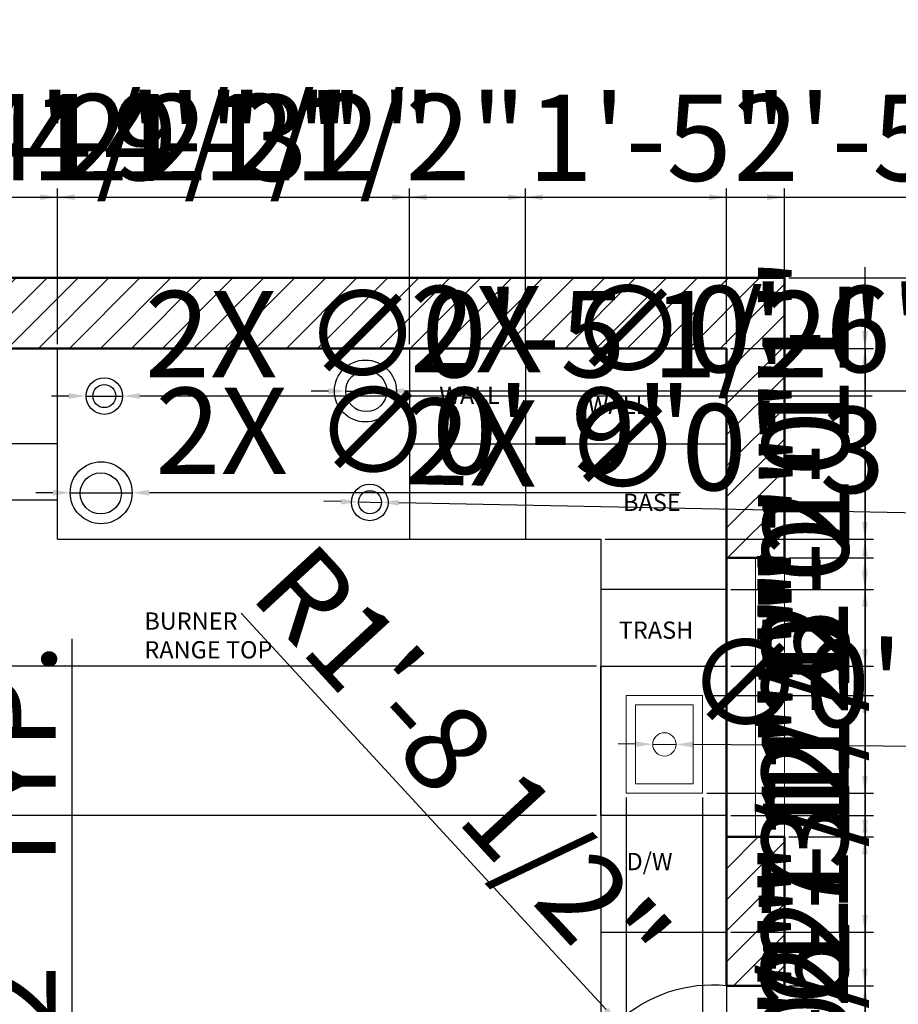
# Model space of a CAD drawing. Units: inches. Extents: x 1545 to 1898, y 1984 to 2198.
# Tile 3 of 4: x 1649 to 1777, y 2055 to 2198. Entities that reach past the tile are written whole.
import ezdxf

# ---------------------------------------------------------------- set-up
doc = ezdxf.new("R2010")
doc.units = ezdxf.units.IN
for name, color, linetype, lineweight in [('A-ANNO-DIMS', 2, 'Continuous', 18), ('A-ANNO-TEXT', 7, 'Continuous', 18), ('A-DOOR', 4, 'Continuous', 25), ('A-EQPM', 9, 'Continuous', 25), ('A-FLOR-CASE', 8, 'Continuous', 25), ('A-FLOR-FIXT', 8, 'Continuous', 18), ('A-GLAZ', 4, 'Continuous', 18), ('A-WALL', 7, 'Continuous', 50), ('A-WALL-PATT', 252, 'Continuous', 13)]:
    doc.layers.add(name, color=color, linetype=linetype, lineweight=lineweight)
doc.styles.get("Standard").update_dxf_attribs({"font": 'arial.ttf'})
doc.dimstyles.new('ISO-25', dxfattribs={"dimtxt": 12.5, "dimasz": 2.5, "dimexe": 1.25, "dimexo": 0.625, "dimtad": 1, "dimdec": 0, "dimlunit": 3, "dimtxsty": 'Standard', "dimcen": 2.5, "dimadec": 0, "dimazin": 0, "dimtfac": 1, "dimtdec": 0, "dimtmove": 0, "dimatfit": 3, "dimfxl": 1, "dimarcsym": 0})

# ---------------------------------------------------------------- blocks, each defined once
blk = doc.blocks.new('*D5')
at = {"layer": 'A-ANNO-DIMS', "color": 0, "lineweight": -2, "transparency": 16777216}
for p, q in [((1760.62, 2160.51), (1812.93, 2160.51)), ((1811.68, 2158.01), (1811.68, 2019.01)), ((1760.62, 2016.51), (1812.93, 2016.51))]:
    blk.add_line(p, q, dxfattribs=at)
at = {"layer": 'A-ANNO-DIMS', "color": 0, "transparency": 16777216}
for points in [[(1811.27, 2158.01), (1812.1, 2158.01), (1811.68, 2160.51)], [(1811.27, 2019.01), (1812.1, 2019.01), (1811.68, 2016.51)]]:
    blk.add_solid(points, dxfattribs=at)
at = {"layer": 'Defpoints', "color": 0, "transparency": 16777216}
for p in [(1759.99, 2160.51), (1759.99, 2016.51), (1811.68, 2016.51)]:
    blk.add_point(p, dxfattribs=at)
at = {"layer": 'A-ANNO-DIMS', "color": 0, "transparency": 16777216, "insert": (1804.78, 2088.51), "char_height": 12.5, "attachment_point": 5, "rotation": 90}
blk.add_mtext("12'", dxfattribs=at)
blk = doc.blocks.new('*D7')
at = {"layer": 'A-ANNO-DIMS', "color": 0, "lineweight": -2, "transparency": 16777216}
for p, q in [((1657.6, 2026.41), (1657.6, 2027.87)), ((1663.11, 2026.41), (1663.11, 2027.87)), ((1655.1, 2026.62), (1652.6, 2026.62)), ((1657.6, 2026.62), (1663.11, 2026.62)), ((1665.61, 2026.62), (1897.84, 2026.62))]:
    blk.add_line(p, q, dxfattribs=at)
at = {"layer": 'A-ANNO-DIMS', "color": 0, "transparency": 16777216}
for points in [[(1655.1, 2027.03), (1655.1, 2026.2), (1657.6, 2026.62)], [(1665.61, 2027.03), (1665.61, 2026.2), (1663.11, 2026.62)]]:
    blk.add_solid(points, dxfattribs=at)
at = {"layer": 'Defpoints', "color": 0, "transparency": 16777216}
for p in [(1663.11, 2026.62), (1657.6, 2025.79), (1663.11, 2025.79)]:
    blk.add_point(p, dxfattribs=at)
at = {"layer": 'A-ANNO-DIMS', "color": 0, "transparency": 16777216, "insert": (1782.98, 2033.7), "char_height": 12.5, "attachment_point": 5}
blk.add_mtext('SCREEN UNIT 0\'-5 1/2" TYP.', dxfattribs=at)
blk = doc.blocks.new('*D8')
at = {"layer": 'A-ANNO-DIMS', "color": 0, "lineweight": -2, "transparency": 16777216}
for p, q in [((1656.77, 2028.29), (1656.77, 2108.23)), ((1656.97, 2025.79), (1655.52, 2025.79)), ((1656.77, 2023.8), (1656.77, 2025.79)), ((1656.97, 2023.8), (1655.52, 2023.8)), ((1656.77, 2021.3), (1656.77, 2018.8))]:
    blk.add_line(p, q, dxfattribs=at)
at = {"layer": 'A-ANNO-DIMS', "color": 0, "transparency": 16777216}
for points in [[(1656.35, 2028.29), (1657.19, 2028.29), (1656.77, 2025.79)], [(1656.35, 2021.3), (1657.19, 2021.3), (1656.77, 2023.8)]]:
    blk.add_solid(points, dxfattribs=at)
at = {"layer": 'Defpoints', "color": 0, "transparency": 16777216}
for p in [(1656.77, 2025.79), (1657.6, 2025.79), (1657.6, 2023.8)]:
    blk.add_point(p, dxfattribs=at)
at = {"layer": 'A-ANNO-DIMS', "color": 0, "transparency": 16777216, "insert": (1649.76, 2069.51), "char_height": 12.5, "attachment_point": 5, "rotation": 90}
blk.add_mtext('0\'-2" TYP.', dxfattribs=at)
blk = doc.blocks.new('*D9')
at = {"layer": 'A-ANNO-DIMS', "color": 0, "lineweight": -2, "transparency": 16777216}
for p, q in [((1582.53, 2161.13), (1582.53, 2173.44)), ((1759.99, 2161.13), (1759.99, 2173.44)), ((1585.03, 2172.19), (1757.49, 2172.19))]:
    blk.add_line(p, q, dxfattribs=at)
at = {"layer": 'A-ANNO-DIMS', "color": 0, "transparency": 16777216}
for points in [[(1585.03, 2172.61), (1585.03, 2171.78), (1582.53, 2172.19)], [(1757.49, 2172.61), (1757.49, 2171.78), (1759.99, 2172.19)]]:
    blk.add_solid(points, dxfattribs=at)
at = {"layer": 'Defpoints', "color": 0, "transparency": 16777216}
for p in [(1759.99, 2172.19), (1582.53, 2160.51), (1759.99, 2160.51)]:
    blk.add_point(p, dxfattribs=at)
at = {"layer": 'A-ANNO-DIMS', "color": 0, "transparency": 16777216, "insert": (1671.26, 2179.28), "char_height": 12.5, "attachment_point": 5}
blk.add_mtext('14\'-9 1/2"', dxfattribs=at)
blk = doc.blocks.new('*D10')
at = {"layer": 'A-ANNO-DIMS', "color": 0, "lineweight": -2, "transparency": 16777216}
for p, q in [((1760.62, 2119.93), (1772.93, 2119.93)), ((1771.68, 2117.43), (1771.68, 2082)), ((1760.62, 2079.5), (1772.93, 2079.5)), ((1771.68, 2079.5), (1771.68, 2013.4))]:
    blk.add_line(p, q, dxfattribs=at)
at = {"layer": 'A-ANNO-DIMS', "color": 0, "transparency": 16777216}
for points in [[(1771.26, 2117.43), (1772.09, 2117.43), (1771.68, 2119.93)], [(1771.26, 2082), (1772.09, 2082), (1771.68, 2079.5)]]:
    blk.add_solid(points, dxfattribs=at)
at = {"layer": 'Defpoints', "color": 0, "transparency": 16777216}
for p in [(1759.99, 2119.93), (1759.99, 2079.5), (1771.68, 2079.5)]:
    blk.add_point(p, dxfattribs=at)
at = {"layer": 'A-ANNO-DIMS', "color": 0, "transparency": 16777216, "insert": (1764.58, 2045.2), "char_height": 12.5, "attachment_point": 5, "rotation": 90}
blk.add_mtext('3\'-4 1/2"', dxfattribs=at)
blk = doc.blocks.new('*D11')
at = {"layer": 'A-ANNO-DIMS', "color": 0, "lineweight": -2, "transparency": 16777216}
for p, q in [((1760.62, 2079.5), (1772.93, 2079.5)), ((1771.68, 2077), (1771.68, 2060.44)), ((1760.62, 2057.94), (1772.93, 2057.94)), ((1771.68, 2057.94), (1771.68, 1993.01))]:
    blk.add_line(p, q, dxfattribs=at)
at = {"layer": 'A-ANNO-DIMS', "color": 0, "transparency": 16777216}
for points in [[(1771.26, 2077), (1772.09, 2077), (1771.68, 2079.5)], [(1771.26, 2060.44), (1772.09, 2060.44), (1771.68, 2057.94)]]:
    blk.add_solid(points, dxfattribs=at)
at = {"layer": 'Defpoints', "color": 0, "transparency": 16777216}
for p in [(1759.99, 2079.5), (1759.99, 2057.94), (1771.68, 2057.94)]:
    blk.add_point(p, dxfattribs=at)
at = {"layer": 'A-ANNO-DIMS', "color": 0, "transparency": 16777216, "insert": (1764.59, 2024.22), "char_height": 12.5, "attachment_point": 5, "rotation": 90}
blk.add_mtext('1\'-9 1/2"', dxfattribs=at)
blk = doc.blocks.new('*D12')
at = {"layer": 'A-ANNO-DIMS', "color": 0, "lineweight": -2, "transparency": 16777216}
for p, q in [((1771.68, 2057.94), (1771.68, 2103.45)), ((1760.62, 2057.94), (1772.93, 2057.94)), ((1771.68, 2037.4), (1771.68, 2055.44)), ((1760.62, 2034.9), (1772.93, 2034.9))]:
    blk.add_line(p, q, dxfattribs=at)
at = {"layer": 'A-ANNO-DIMS', "color": 0, "transparency": 16777216}
for points in [[(1771.26, 2055.44), (1772.09, 2055.44), (1771.68, 2057.94)], [(1771.26, 2037.4), (1772.09, 2037.4), (1771.68, 2034.9)]]:
    blk.add_solid(points, dxfattribs=at)
at = {"layer": 'Defpoints', "color": 0, "transparency": 16777216}
for p in [(1759.99, 2057.94), (1771.68, 2057.94), (1759.99, 2034.9)]:
    blk.add_point(p, dxfattribs=at)
at = {"layer": 'A-ANNO-DIMS', "color": 0, "transparency": 16777216, "insert": (1764.78, 2081.94), "char_height": 12.5, "attachment_point": 5, "rotation": 90}
blk.add_mtext('1\'-11"', dxfattribs=at)
blk = doc.blocks.new('*D13')
at = {"layer": 'A-ANNO-DIMS', "color": 0, "lineweight": -2, "transparency": 16777216}
for p, q in [((1771.68, 2034.9), (1771.68, 2099.83)), ((1760.62, 2034.9), (1772.93, 2034.9)), ((1771.68, 2019.01), (1771.68, 2032.4)), ((1760.62, 2016.51), (1772.93, 2016.51))]:
    blk.add_line(p, q, dxfattribs=at)
at = {"layer": 'A-ANNO-DIMS', "color": 0, "transparency": 16777216}
for points in [[(1771.26, 2032.4), (1772.09, 2032.4), (1771.68, 2034.9)], [(1771.26, 2019.01), (1772.09, 2019.01), (1771.68, 2016.51)]]:
    blk.add_solid(points, dxfattribs=at)
at = {"layer": 'Defpoints', "color": 0, "transparency": 16777216}
for p in [(1759.99, 2034.9), (1771.68, 2034.9), (1759.99, 2016.51)]:
    blk.add_point(p, dxfattribs=at)
at = {"layer": 'A-ANNO-DIMS', "color": 0, "transparency": 16777216, "insert": (1764.59, 2068.62), "char_height": 12.5, "attachment_point": 5, "rotation": 90}
blk.add_mtext('1\'-6 1/2"', dxfattribs=at)
blk = doc.blocks.new('*D16')
at = {"layer": 'A-ANNO-DIMS', "color": 0, "lineweight": -2, "transparency": 16777216}
for p, q in [((1760.62, 2160.51), (1772.93, 2160.51)), ((1771.68, 2158.01), (1771.68, 2152.8)), ((1752.23, 2150.3), (1772.93, 2150.3)), ((1771.68, 2150.3), (1771.68, 2103.61))]:
    blk.add_line(p, q, dxfattribs=at)
at = {"layer": 'A-ANNO-DIMS', "color": 0, "transparency": 16777216}
for points in [[(1771.26, 2158.01), (1772.09, 2158.01), (1771.68, 2160.51)], [(1771.26, 2152.8), (1772.09, 2152.8), (1771.68, 2150.3)]]:
    blk.add_solid(points, dxfattribs=at)
at = {"layer": 'Defpoints', "color": 0, "transparency": 16777216}
for p in [(1759.99, 2160.51), (1751.61, 2150.3), (1771.68, 2150.3)]:
    blk.add_point(p, dxfattribs=at)
at = {"layer": 'A-ANNO-DIMS', "color": 0, "transparency": 16777216, "insert": (1764.67, 2125.71), "char_height": 12.5, "attachment_point": 5, "rotation": 90}
blk.add_mtext('0\'-10"', dxfattribs=at)
blk = doc.blocks.new('*D22')
at = {"layer": 'A-ANNO-DIMS', "color": 0, "lineweight": -2, "transparency": 16777216}
for p, q in [((1600.47, 2150.93), (1600.47, 2173.44)), ((1629.21, 2150.93), (1629.21, 2173.44)), ((1602.97, 2172.19), (1626.71, 2172.19)), ((1629.21, 2172.19), (1695.52, 2172.19))]:
    blk.add_line(p, q, dxfattribs=at)
at = {"layer": 'A-ANNO-DIMS', "color": 0, "transparency": 16777216}
for points in [[(1602.97, 2172.61), (1602.97, 2171.78), (1600.47, 2172.19)], [(1626.71, 2172.61), (1626.71, 2171.78), (1629.21, 2172.19)]]:
    blk.add_solid(points, dxfattribs=at)
at = {"layer": 'Defpoints', "color": 0, "transparency": 16777216}
for p in [(1629.21, 2172.19), (1600.47, 2150.3), (1629.21, 2150.3)]:
    blk.add_point(p, dxfattribs=at)
at = {"layer": 'A-ANNO-DIMS', "color": 0, "transparency": 16777216, "insert": (1663.61, 2179.28), "char_height": 12.5, "attachment_point": 5}
blk.add_mtext('2\'-4 1/2"', dxfattribs=at)
blk = doc.blocks.new('*D23')
at = {"layer": 'A-ANNO-DIMS', "color": 0, "lineweight": -2, "transparency": 16777216}
for p, q in [((1629.21, 2150.93), (1629.21, 2173.44)), ((1654.65, 2150.93), (1654.65, 2173.44)), ((1631.71, 2172.19), (1652.15, 2172.19)), ((1654.65, 2172.19), (1720.96, 2172.19))]:
    blk.add_line(p, q, dxfattribs=at)
at = {"layer": 'A-ANNO-DIMS', "color": 0, "transparency": 16777216}
for points in [[(1631.71, 2172.61), (1631.71, 2171.78), (1629.21, 2172.19)], [(1652.15, 2172.61), (1652.15, 2171.78), (1654.65, 2172.19)]]:
    blk.add_solid(points, dxfattribs=at)
at = {"layer": 'Defpoints', "color": 0, "transparency": 16777216}
for p in [(1654.65, 2172.19), (1629.21, 2150.3), (1654.65, 2150.3)]:
    blk.add_point(p, dxfattribs=at)
at = {"layer": 'A-ANNO-DIMS', "color": 0, "transparency": 16777216, "insert": (1689.05, 2179.28), "char_height": 12.5, "attachment_point": 5}
blk.add_mtext('2\'-1 1/2"', dxfattribs=at)
blk = doc.blocks.new('*D24')
at = {"layer": 'A-ANNO-DIMS', "color": 0, "lineweight": -2, "transparency": 16777216}
for p, q in [((1654.65, 2150.93), (1654.65, 2173.44)), ((1705.66, 2150.93), (1705.66, 2173.44)), ((1657.15, 2172.19), (1703.16, 2172.19))]:
    blk.add_line(p, q, dxfattribs=at)
at = {"layer": 'A-ANNO-DIMS', "color": 0, "transparency": 16777216}
for points in [[(1657.15, 2172.61), (1657.15, 2171.78), (1654.65, 2172.19)], [(1703.16, 2172.61), (1703.16, 2171.78), (1705.66, 2172.19)]]:
    blk.add_solid(points, dxfattribs=at)
at = {"layer": 'Defpoints', "color": 0, "transparency": 16777216}
for p in [(1705.66, 2172.19), (1654.65, 2150.3), (1705.66, 2150.3)]:
    blk.add_point(p, dxfattribs=at)
at = {"layer": 'A-ANNO-DIMS', "color": 0, "transparency": 16777216, "insert": (1680.15, 2179.2), "char_height": 12.5, "attachment_point": 5}
blk.add_mtext('4\'-3"', dxfattribs=at)
blk = doc.blocks.new('*D25')
at = {"layer": 'A-ANNO-DIMS', "color": 0, "lineweight": -2, "transparency": 16777216}
for p, q in [((1705.66, 2150.93), (1705.66, 2173.44)), ((1722.46, 2150.93), (1722.46, 2173.44)), ((1708.16, 2172.19), (1719.96, 2172.19)), ((1722.46, 2172.19), (1758.26, 2172.19))]:
    blk.add_line(p, q, dxfattribs=at)
at = {"layer": 'A-ANNO-DIMS', "color": 0, "transparency": 16777216}
for points in [[(1708.16, 2172.61), (1708.16, 2171.78), (1705.66, 2172.19)], [(1719.96, 2172.61), (1719.96, 2171.78), (1722.46, 2172.19)]]:
    blk.add_solid(points, dxfattribs=at)
at = {"layer": 'Defpoints', "color": 0, "transparency": 16777216}
for p in [(1722.46, 2172.19), (1705.66, 2150.3), (1722.46, 2150.3)]:
    blk.add_point(p, dxfattribs=at)
at = {"layer": 'A-ANNO-DIMS', "color": 0, "transparency": 16777216, "insert": (1741.61, 2179.2), "char_height": 12.5, "attachment_point": 5}
blk.add_mtext('1\'-5"', dxfattribs=at)
blk = doc.blocks.new('*D26')
at = {"layer": 'A-ANNO-DIMS', "color": 0, "lineweight": -2, "transparency": 16777216}
for p, q in [((1722.46, 2150.93), (1722.46, 2173.44)), ((1751.61, 2150.93), (1751.61, 2173.44)), ((1724.96, 2172.19), (1749.11, 2172.19)), ((1751.61, 2172.19), (1788.8, 2172.19))]:
    blk.add_line(p, q, dxfattribs=at)
at = {"layer": 'A-ANNO-DIMS', "color": 0, "transparency": 16777216}
for points in [[(1724.96, 2172.61), (1724.96, 2171.78), (1722.46, 2172.19)], [(1749.11, 2172.61), (1749.11, 2171.78), (1751.61, 2172.19)]]:
    blk.add_solid(points, dxfattribs=at)
at = {"layer": 'Defpoints', "color": 0, "transparency": 16777216}
for p in [(1751.61, 2172.19), (1722.46, 2150.3), (1751.61, 2150.3)]:
    blk.add_point(p, dxfattribs=at)
at = {"layer": 'A-ANNO-DIMS', "color": 0, "transparency": 16777216, "insert": (1771.45, 2179.2), "char_height": 12.5, "attachment_point": 5}
blk.add_mtext('2\'-5"', dxfattribs=at)
blk = doc.blocks.new('*D31')
at = {"layer": 'A-ANNO-DIMS', "color": 0, "lineweight": -2, "transparency": 16777216}
for p, q in [((1752.23, 2150.3), (1772.93, 2150.3)), ((1771.68, 2147.8), (1771.68, 2125.15)), ((1734.02, 2122.65), (1772.93, 2122.65)), ((1771.68, 2122.65), (1771.68, 2056.33))]:
    blk.add_line(p, q, dxfattribs=at)
at = {"layer": 'A-ANNO-DIMS', "color": 0, "transparency": 16777216}
for points in [[(1771.26, 2147.8), (1772.09, 2147.8), (1771.68, 2150.3)], [(1771.26, 2125.15), (1772.09, 2125.15), (1771.68, 2122.65)]]:
    blk.add_solid(points, dxfattribs=at)
at = {"layer": 'Defpoints', "color": 0, "transparency": 16777216}
for p in [(1751.61, 2150.3), (1733.39, 2122.65), (1771.68, 2122.65)]:
    blk.add_point(p, dxfattribs=at)
at = {"layer": 'A-ANNO-DIMS', "color": 0, "transparency": 16777216, "insert": (1764.58, 2088.24), "char_height": 12.5, "attachment_point": 5, "rotation": 90}
blk.add_mtext('2\'-3 1/2"', dxfattribs=at)
blk = doc.blocks.new('*D32')
at = {"layer": 'A-ANNO-DIMS', "color": 0, "lineweight": -2, "transparency": 16777216}
for p, q in [((1734.02, 2122.65), (1772.93, 2122.65)), ((1771.68, 2120.15), (1771.68, 2117.88)), ((1752.23, 2115.38), (1772.93, 2115.38)), ((1771.68, 2115.38), (1771.68, 2049.27))]:
    blk.add_line(p, q, dxfattribs=at)
at = {"layer": 'A-ANNO-DIMS', "color": 0, "transparency": 16777216}
for points in [[(1771.26, 2120.15), (1772.09, 2120.15), (1771.68, 2122.65)], [(1771.26, 2117.88), (1772.09, 2117.88), (1771.68, 2115.38)]]:
    blk.add_solid(points, dxfattribs=at)
at = {"layer": 'Defpoints', "color": 0, "transparency": 16777216}
for p in [(1733.39, 2122.65), (1751.61, 2115.38), (1771.68, 2115.38)]:
    blk.add_point(p, dxfattribs=at)
at = {"layer": 'A-ANNO-DIMS', "color": 0, "transparency": 16777216, "insert": (1764.59, 2081.08), "char_height": 12.5, "attachment_point": 5, "rotation": 90}
blk.add_mtext('0\'-7 1/2"', dxfattribs=at)
blk = doc.blocks.new('*D33')
at = {"layer": 'A-ANNO-DIMS', "color": 0, "lineweight": -2, "transparency": 16777216}
for p, q in [((1771.68, 2082.61), (1771.68, 2118.41)), ((1752.23, 2082.61), (1772.93, 2082.61)), ((1771.68, 2068.2), (1771.68, 2080.11)), ((1752.23, 2065.7), (1772.93, 2065.7))]:
    blk.add_line(p, q, dxfattribs=at)
at = {"layer": 'A-ANNO-DIMS', "color": 0, "transparency": 16777216}
for points in [[(1771.26, 2080.11), (1772.09, 2080.11), (1771.68, 2082.61)], [(1771.26, 2068.2), (1772.09, 2068.2), (1771.68, 2065.7)]]:
    blk.add_solid(points, dxfattribs=at)
at = {"layer": 'Defpoints', "color": 0, "transparency": 16777216}
for p in [(1751.61, 2082.61), (1771.68, 2082.61), (1751.61, 2065.7)]:
    blk.add_point(p, dxfattribs=at)
at = {"layer": 'A-ANNO-DIMS', "color": 0, "transparency": 16777216, "insert": (1764.67, 2101.76), "char_height": 12.5, "attachment_point": 5, "rotation": 90}
blk.add_mtext('1\'-5"', dxfattribs=at)
blk = doc.blocks.new('*D34')
at = {"layer": 'A-ANNO-DIMS', "color": 0, "lineweight": -2, "transparency": 16777216}
for p, q in [((1570.84, 2104.25), (1570.84, 2169.18)), ((1732.77, 2104.25), (1569.59, 2104.25)), ((1570.84, 2085.11), (1570.84, 2101.75)), ((1732.77, 2082.61), (1569.59, 2082.61))]:
    blk.add_line(p, q, dxfattribs=at)
at = {"layer": 'A-ANNO-DIMS', "color": 0, "transparency": 16777216}
for points in [[(1570.42, 2101.75), (1571.26, 2101.75), (1570.84, 2104.25)], [(1570.42, 2085.11), (1571.26, 2085.11), (1570.84, 2082.61)]]:
    blk.add_solid(points, dxfattribs=at)
at = {"layer": 'Defpoints', "color": 0, "transparency": 16777216}
for p in [(1570.84, 2104.25), (1733.39, 2104.25), (1733.39, 2082.61)]:
    blk.add_point(p, dxfattribs=at)
at = {"layer": 'A-ANNO-DIMS', "color": 0, "transparency": 16777216, "insert": (1563.75, 2137.96), "char_height": 12.5, "attachment_point": 5, "rotation": 90}
blk.add_mtext('1\'-9 1/2"', dxfattribs=at)
blk = doc.blocks.new('*D35')
at = {"layer": 'A-ANNO-DIMS', "color": 0, "lineweight": -2, "transparency": 16777216}
for p, q in [((1771.68, 2115.38), (1771.68, 2162.07)), ((1752.23, 2115.38), (1772.93, 2115.38)), ((1771.68, 2106.75), (1771.68, 2112.88)), ((1752.23, 2104.25), (1772.93, 2104.25))]:
    blk.add_line(p, q, dxfattribs=at)
at = {"layer": 'A-ANNO-DIMS', "color": 0, "transparency": 16777216}
for points in [[(1771.26, 2112.88), (1772.09, 2112.88), (1771.68, 2115.38)], [(1771.26, 2106.75), (1772.09, 2106.75), (1771.68, 2104.25)]]:
    blk.add_solid(points, dxfattribs=at)
at = {"layer": 'Defpoints', "color": 0, "transparency": 16777216}
for p in [(1751.61, 2115.38), (1771.68, 2115.38), (1751.61, 2104.25)]:
    blk.add_point(p, dxfattribs=at)
at = {"layer": 'A-ANNO-DIMS', "color": 0, "transparency": 16777216, "insert": (1764.67, 2139.97), "char_height": 12.5, "attachment_point": 5, "rotation": 90}
blk.add_mtext('0\'-11"', dxfattribs=at)
blk = doc.blocks.new('*D36')
at = {"layer": 'A-ANNO-DIMS', "color": 0, "lineweight": -2, "transparency": 16777216}
for p, q in [((1600.47, 2063.41), (1600.47, 2003.57)), ((1630.49, 2063.41), (1630.49, 2003.57)), ((1602.97, 2004.82), (1627.99, 2004.82)), ((1630.49, 2004.82), (1667.68, 2004.82))]:
    blk.add_line(p, q, dxfattribs=at)
at = {"layer": 'A-ANNO-DIMS', "color": 0, "transparency": 16777216}
for points in [[(1602.97, 2005.24), (1602.97, 2004.41), (1600.47, 2004.82)], [(1627.99, 2005.24), (1627.99, 2004.41), (1630.49, 2004.82)]]:
    blk.add_solid(points, dxfattribs=at)
at = {"layer": 'Defpoints', "color": 0, "transparency": 16777216}
for p in [(1600.47, 2064.03), (1630.49, 2064.03), (1630.49, 2004.82)]:
    blk.add_point(p, dxfattribs=at)
at = {"layer": 'A-ANNO-DIMS', "color": 0, "transparency": 16777216, "insert": (1650.33, 2011.83), "char_height": 12.5, "attachment_point": 5}
blk.add_mtext('2\'-6"', dxfattribs=at)
blk = doc.blocks.new('*D37')
at = {"layer": 'A-ANNO-DIMS', "color": 0, "lineweight": -2, "transparency": 16777216}
for p, q in [((1733.39, 2065.08), (1733.39, 2003.57)), ((1751.61, 2065.08), (1751.61, 2003.57)), ((1735.89, 2004.82), (1749.11, 2004.82)), ((1751.61, 2004.82), (1787.41, 2004.82))]:
    blk.add_line(p, q, dxfattribs=at)
at = {"layer": 'A-ANNO-DIMS', "color": 0, "transparency": 16777216}
for points in [[(1735.89, 2005.24), (1735.89, 2004.41), (1733.39, 2004.82)], [(1749.11, 2005.24), (1749.11, 2004.41), (1751.61, 2004.82)]]:
    blk.add_solid(points, dxfattribs=at)
at = {"layer": 'Defpoints', "color": 0, "transparency": 16777216}
for p in [(1733.39, 2065.7), (1751.61, 2065.7), (1751.61, 2004.82)]:
    blk.add_point(p, dxfattribs=at)
at = {"layer": 'A-ANNO-DIMS', "color": 0, "transparency": 16777216, "insert": (1770.76, 2011.83), "char_height": 12.5, "attachment_point": 5}
blk.add_mtext('1\'-6"', dxfattribs=at)
blk = doc.blocks.new('*D38')
at = {"layer": 'A-ANNO-DIMS', "color": 0, "lineweight": -2, "transparency": 16777216}
for p, q in [((1627.57, 2127.73), (1627.57, 2003.57)), ((1733.39, 2122.03), (1733.39, 2003.57)), ((1630.07, 2004.82), (1730.89, 2004.82))]:
    blk.add_line(p, q, dxfattribs=at)
at = {"layer": 'A-ANNO-DIMS', "color": 0, "transparency": 16777216}
for points in [[(1630.07, 2005.24), (1630.07, 2004.41), (1627.57, 2004.82)], [(1730.89, 2005.24), (1730.89, 2004.41), (1733.39, 2004.82)]]:
    blk.add_solid(points, dxfattribs=at)
at = {"layer": 'Defpoints', "color": 0, "transparency": 16777216}
for p in [(1627.57, 2128.35), (1733.39, 2122.65), (1733.39, 2004.82)]:
    blk.add_point(p, dxfattribs=at)
at = {"layer": 'A-ANNO-DIMS', "color": 0, "transparency": 16777216, "insert": (1680.48, 2011.83), "char_height": 12.5, "attachment_point": 5}
blk.add_mtext('8\'-10"', dxfattribs=at)
blk = doc.blocks.new('*D40')
at = {"layer": 'A-ANNO-DIMS', "color": 0, "lineweight": -2, "transparency": 16777216}
for p, q in [((1600.47, 2084.8), (1600.47, 2173.44)), ((1617.18, 2084.8), (1617.18, 2173.44)), ((1602.97, 2172.19), (1614.68, 2172.19)), ((1617.18, 2172.19), (1682.11, 2172.19))]:
    blk.add_line(p, q, dxfattribs=at)
at = {"layer": 'A-ANNO-DIMS', "color": 0, "transparency": 16777216}
for points in [[(1602.97, 2172.61), (1602.97, 2171.78), (1600.47, 2172.19)], [(1614.68, 2172.61), (1614.68, 2171.78), (1617.18, 2172.19)]]:
    blk.add_solid(points, dxfattribs=at)
at = {"layer": 'Defpoints', "color": 0, "transparency": 16777216}
for p in [(1617.18, 2172.19), (1600.47, 2084.18), (1617.18, 2084.18)]:
    blk.add_point(p, dxfattribs=at)
at = {"layer": 'A-ANNO-DIMS', "color": 0, "transparency": 16777216, "insert": (1650.89, 2179.28), "char_height": 12.5, "attachment_point": 5}
blk.add_mtext('1\'-4 1/2"', dxfattribs=at)
blk = doc.blocks.new('*D41')
at = {"layer": 'A-ANNO-DIMS', "color": 0, "lineweight": -2, "transparency": 16777216}
for p, q in [((1737.08, 2085.23), (1737.08, 2003.57)), ((1748.11, 2085.23), (1748.11, 2003.57)), ((1739.58, 2004.82), (1745.61, 2004.82)), ((1748.11, 2004.82), (1794.8, 2004.82))]:
    blk.add_line(p, q, dxfattribs=at)
at = {"layer": 'A-ANNO-DIMS', "color": 0, "transparency": 16777216}
for points in [[(1739.58, 2005.24), (1739.58, 2004.41), (1737.08, 2004.82)], [(1745.61, 2005.24), (1745.61, 2004.41), (1748.11, 2004.82)]]:
    blk.add_solid(points, dxfattribs=at)
at = {"layer": 'Defpoints', "color": 0, "transparency": 16777216}
for p in [(1737.08, 2085.86), (1748.11, 2085.86), (1748.11, 2004.82)]:
    blk.add_point(p, dxfattribs=at)
at = {"layer": 'A-ANNO-DIMS', "color": 0, "transparency": 16777216, "insert": (1772.71, 2011.83), "char_height": 12.5, "attachment_point": 5}
blk.add_mtext('0\'-11"', dxfattribs=at)
blk = doc.blocks.new('*D42')
at = {"layer": 'A-ANNO-DIMS', "color": 0, "lineweight": -2, "transparency": 16777216}
for p, q in [((1771.68, 2099.99), (1771.68, 2135.79)), ((1748.74, 2099.99), (1772.93, 2099.99)), ((1771.68, 2088.36), (1771.68, 2097.49)), ((1748.74, 2085.86), (1772.93, 2085.86))]:
    blk.add_line(p, q, dxfattribs=at)
at = {"layer": 'A-ANNO-DIMS', "color": 0, "transparency": 16777216}
for points in [[(1771.26, 2097.49), (1772.09, 2097.49), (1771.68, 2099.99)], [(1771.26, 2088.36), (1772.09, 2088.36), (1771.68, 2085.86)]]:
    blk.add_solid(points, dxfattribs=at)
at = {"layer": 'Defpoints', "color": 0, "transparency": 16777216}
for p in [(1748.11, 2099.99), (1771.68, 2099.99), (1748.11, 2085.86)]:
    blk.add_point(p, dxfattribs=at)
at = {"layer": 'A-ANNO-DIMS', "color": 0, "transparency": 16777216, "insert": (1764.78, 2119.14), "char_height": 12.5, "attachment_point": 5, "rotation": 90}
blk.add_mtext('1\'-2"', dxfattribs=at)
blk = doc.blocks.new('*D43')
at = {"layer": 'A-ANNO-DIMS', "color": 0, "lineweight": -2, "transparency": 16777216}
for p, q in [((1681.27, 2111.93), (1734.16, 2054.51)), ((1749.6, 2037.74), (1735.85, 2052.67))]:
    blk.add_line(p, q, dxfattribs=at)
at = {"layer": 'A-ANNO-DIMS', "color": 0, "transparency": 16777216}
blk.add_solid([(1734.46, 2054.79), (1733.85, 2054.22), (1735.85, 2052.67)], dxfattribs=at)
at = {"layer": 'Defpoints', "color": 0, "transparency": 16777216}
for p in [(1735.85, 2052.67), (1749.6, 2037.74)]:
    blk.add_point(p, dxfattribs=at)
at = {"layer": 'A-ANNO-DIMS', "color": 0, "transparency": 16777216, "insert": (1712.08, 2088.94), "char_height": 12.5, "attachment_point": 5, "rotation": 312.6451}
blk.add_mtext('R1\'-8 1/2"', dxfattribs=at)
blk = doc.blocks.new('*D44')
at = {"layer": 'A-ANNO-DIMS', "color": 0, "lineweight": -2, "transparency": 16777216}
for p, q in [((1653.98, 2129.38), (1651.48, 2129.38)), ((1656.48, 2129.38), (1665.46, 2129.38)), ((1744.95, 2129.39), (1667.96, 2129.38))]:
    blk.add_line(p, q, dxfattribs=at)
at = {"layer": 'A-ANNO-DIMS', "color": 0, "transparency": 16777216}
for points in [[(1653.98, 2129.8), (1653.98, 2128.97), (1656.48, 2129.38)], [(1667.96, 2129.8), (1667.96, 2128.97), (1665.46, 2129.38)]]:
    blk.add_solid(points, dxfattribs=at)
at = {"layer": 'Defpoints', "color": 0, "transparency": 16777216}
for p in [(1656.48, 2129.38), (1665.46, 2129.38)]:
    blk.add_point(p, dxfattribs=at)
at = {"layer": 'A-ANNO-DIMS', "color": 0, "transparency": 16777216, "insert": (1707.71, 2136.74), "char_height": 12.5, "attachment_point": 5, "rotation": 0.005}
blk.add_mtext('2X ∅0\'-9"', dxfattribs=at)
blk = doc.blocks.new('*D45')
at = {"layer": 'A-ANNO-DIMS', "color": 0, "lineweight": -2, "transparency": 16777216}
for p, q in [((1693.9, 2144.11), (1691.4, 2144.11)), ((1696.4, 2144.11), (1702.37, 2144.11)), ((1781.85, 2144.11), (1704.87, 2144.11))]:
    blk.add_line(p, q, dxfattribs=at)
at = {"layer": 'A-ANNO-DIMS', "color": 0, "transparency": 16777216}
for points in [[(1693.9, 2144.53), (1693.9, 2143.7), (1696.4, 2144.11)], [(1704.87, 2144.53), (1704.87, 2143.7), (1702.37, 2144.11)]]:
    blk.add_solid(points, dxfattribs=at)
at = {"layer": 'Defpoints', "color": 0, "transparency": 16777216}
for p in [(1696.4, 2144.11), (1702.37, 2144.11)]:
    blk.add_point(p, dxfattribs=at)
at = {"layer": 'A-ANNO-DIMS', "color": 0, "transparency": 16777216, "insert": (1744.61, 2151.47), "char_height": 12.5, "attachment_point": 5, "rotation": 359.999}
blk.add_mtext('2X ∅0\'-6"', dxfattribs=at)
blk = doc.blocks.new('*D46')
at = {"layer": 'A-ANNO-DIMS', "color": 0, "lineweight": -2, "transparency": 16777216}
for p, q in [((1656.28, 2143.39), (1653.78, 2143.39)), ((1658.78, 2143.39), (1664.08, 2143.39)), ((1772.7, 2143.37), (1666.58, 2143.39))]:
    blk.add_line(p, q, dxfattribs=at)
at = {"layer": 'A-ANNO-DIMS', "color": 0, "transparency": 16777216}
for points in [[(1656.28, 2143.8), (1656.28, 2142.97), (1658.78, 2143.39)], [(1666.58, 2143.8), (1666.58, 2142.97), (1664.08, 2143.39)]]:
    blk.add_solid(points, dxfattribs=at)
at = {"layer": 'Defpoints', "color": 0, "transparency": 16777216}
for p in [(1658.78, 2143.39), (1664.08, 2143.39)]:
    blk.add_point(p, dxfattribs=at)
at = {"layer": 'A-ANNO-DIMS', "color": 0, "transparency": 16777216, "insert": (1720.89, 2150.74), "char_height": 12.5, "attachment_point": 5, "rotation": 359.9927}
blk.add_mtext('2X ∅0\'-5 1/2"', dxfattribs=at)
blk = doc.blocks.new('*D47')
at = {"layer": 'A-ANNO-DIMS', "color": 0, "lineweight": -2, "transparency": 16777216}
for p, q in [((1695.76, 2128.1), (1693.26, 2128.15)), ((1698.26, 2128.05), (1701.6, 2127.98)), ((1810.19, 2125.79), (1704.1, 2127.93))]:
    blk.add_line(p, q, dxfattribs=at)
at = {"layer": 'A-ANNO-DIMS', "color": 0, "transparency": 16777216}
for points in [[(1695.76, 2128.51), (1695.75, 2127.68), (1698.26, 2128.05)], [(1704.11, 2128.35), (1704.09, 2127.51), (1701.6, 2127.98)]]:
    blk.add_solid(points, dxfattribs=at)
at = {"layer": 'Defpoints', "color": 0, "transparency": 16777216}
for p in [(1698.26, 2128.05), (1701.6, 2127.98)]:
    blk.add_point(p, dxfattribs=at)
at = {"layer": 'A-ANNO-DIMS', "color": 0, "transparency": 16777216, "insert": (1758.54, 2134.19), "char_height": 12.5, "attachment_point": 5, "rotation": 358.8454}
blk.add_mtext('2X ∅0\'-3 1/2"', dxfattribs=at)
blk = doc.blocks.new('*D48')
at = {"layer": 'A-ANNO-DIMS', "color": 0, "lineweight": -2, "transparency": 16777216}
for p, q in [((1738.41, 2092.96), (1735.91, 2092.98)), ((1740.91, 2092.94), (1744.28, 2092.91)), ((1826.49, 2092.27), (1746.78, 2092.89))]:
    blk.add_line(p, q, dxfattribs=at)
at = {"layer": 'A-ANNO-DIMS', "color": 0, "transparency": 16777216}
for points in [[(1738.42, 2093.37), (1738.41, 2092.54), (1740.91, 2092.94)], [(1746.79, 2093.31), (1746.78, 2092.47), (1744.28, 2092.91)]]:
    blk.add_solid(points, dxfattribs=at)
at = {"layer": 'Defpoints', "color": 0, "transparency": 16777216}
for p in [(1740.91, 2092.94), (1744.28, 2092.91)]:
    blk.add_point(p, dxfattribs=at)
at = {"layer": 'A-ANNO-DIMS', "color": 0, "transparency": 16777216, "insert": (1787.94, 2099.93), "char_height": 12.5, "attachment_point": 5, "rotation": 359.5524}
blk.add_mtext('∅0\'-3 1/2"', dxfattribs=at)

msp = doc.modelspace()

# ---------------------------------------------------------------- hatches: boundary and pattern name
at = {"layer": 'A-WALL-PATT'}
h = msp.add_hatch(dxfattribs=at)
h.set_pattern_fill('ANSI31', color=256)
h.paths.add_polyline_path([(1759.99, 2160.51), (1639.99, 2160.51), (1582.53, 2160.51), (1582.53, 2150.3), (1591.3, 2150.3), (1591.3, 2056.44), (1600.47, 2056.44), (1600.47, 2150.3), (1751.61, 2150.3), (1751.61, 2119.93), (1759.99, 2119.93)])
h.paths.add_polyline_path([(1759.99, 2079.5), (1751.61, 2079.5), (1751.61, 2057.94), (1759.99, 2057.94)], flags=17)
h.paths.add_polyline_path([(1599.8, 2117.08), (1610.56, 2117.08), (1610.56, 2122.23), (1599.8, 2122.23)], flags=24)

# ---------------------------------------------------------------- linework, layer by layer
at = {"layer": 'A-DOOR'}
msp.add_arc((1749.6, 2037.74), 20.3, 84.3172, 180.9706, dxfattribs=at)
at = {"layer": 'A-EQPM'}
for p, q in [((1654.65, 2122.65), (1705.66, 2122.65)), ((1751.61, 2082.61), (1733.39, 2082.61)), ((1751.61, 2065.7), (1751.61, 2082.61)), ((1733.39, 2065.7), (1751.61, 2065.7))]:
    msp.add_line(p, q, dxfattribs=at)
msp.add_lwpolyline([(1654.65, 2122.65), (1654.65, 2150.3), (1705.66, 2150.3), (1705.66, 2122.65)], dxfattribs=at)
for centre, radius in [((1699.27, 2144.12), 4.49), ((1661.43, 2143.39), 2.65), ((1699.39, 2144.11), 2.98), ((1661.43, 2143.39), 1.67), ((1660.97, 2129.38), 4.49), ((1660.92, 2129.28), 2.98), ((1699.9, 2127.98), 2.65), ((1699.93, 2128.01), 1.67)]:
    msp.add_circle(centre, radius, dxfattribs=at)
at = {"layer": 'A-FLOR-CASE'}
for p, q in [((1722.46, 2150.3), (1722.46, 2122.65)), ((1654.65, 2136.48), (1617.18, 2136.48)), ((1705.66, 2136.48), (1751.61, 2136.48)), ((1627.57, 2128.35), (1654.65, 2128.35)), ((1705.66, 2122.65), (1733.39, 2122.65)), ((1733.39, 2122.65), (1733.39, 2065.7)), ((1751.61, 2115.38), (1733.39, 2115.38)), ((1751.61, 2104.25), (1751.61, 2115.38)), ((1733.39, 2082.61), (1733.39, 2104.25)), ((1733.39, 2104.25), (1751.61, 2104.25))]:
    msp.add_line(p, q, dxfattribs=at)
at = {"layer": 'A-FLOR-FIXT'}
for points in [[(1737.08, 2099.99), (1748.11, 2099.99), (1748.11, 2085.86), (1737.08, 2085.86)], [(1738.42, 2098.63), (1746.79, 2098.63), (1746.79, 2087.21), (1738.42, 2087.21)]]:
    msp.add_lwpolyline(points, close=True, dxfattribs=at)
msp.add_circle((1742.6, 2092.92), 1.69, dxfattribs=at)
at = {"layer": 'A-GLAZ'}
for p, q in [((1751.61, 2079.5), (1751.61, 2119.93)), ((1755.8, 2119.93), (1755.8, 2079.5)), ((1759.99, 2119.93), (1759.99, 2079.5))]:
    msp.add_line(p, q, dxfattribs=at)
at = {"layer": 'A-WALL'}
for p, q in [((1639.99, 2160.51), (1759.99, 2160.51)), ((1759.99, 2160.51), (1759.99, 2119.93)), ((1600.47, 2150.3), (1751.61, 2150.3)), ((1751.61, 2150.3), (1751.61, 2057.94)), ((1751.61, 2119.93), (1759.99, 2119.93)), ((1759.99, 2079.5), (1751.61, 2079.5)), ((1759.99, 2079.5), (1759.99, 2057.94)), ((1759.99, 2057.94), (1751.61, 2057.94))]:
    msp.add_line(p, q, dxfattribs=at)

# ---------------------------------------------------------------- texts
at = {"layer": 'A-ANNO-TEXT', "char_height": 2.5, "attachment_point": 1}
for s, width, insert in [('WALL', 15.901, (1709.97, 2144.74)), ('WALL', 15.901, (1731.5, 2143.3)), ('BASE', 14.4938, (1736.61, 2129.24)), ('BASE', 14.4938, (1736.61, 2129.24)), ('BURNER\\PRANGE TOP', 29.8319, (1667.23, 2112.04)), ('TRASH', 11.673, (1735.99, 2110.72)), ('D/W', 9.6065, (1737.11, 2077.19))]:
    msp.add_mtext_dynamic_manual_height_columns(s, width=width, gutter_width=12.5, heights=[0], dxfattribs=dict(at, insert=insert))

# ---------------------------------------------------------------- dimensions: what is measured, and where the dimension line sits
at = {"layer": 'A-ANNO-DIMS'}
for base, p1, p2, picture, middle in [((1759.99, 2172.19), (1582.53, 2160.51), (1759.99, 2160.51), '*D9', (1671.26, 2179.28)), ((1629.21, 2172.19), (1600.47, 2150.3), (1629.21, 2150.3), '*D22', (1663.61, 2179.28)), ((1617.18, 2172.19), (1600.47, 2084.18), (1617.18, 2084.18), '*D40', (1650.89, 2179.28)), ((1654.65, 2172.19), (1629.21, 2150.3), (1654.65, 2150.3), '*D23', (1689.05, 2179.28)), ((1705.66, 2172.19), (1654.65, 2150.3), (1705.66, 2150.3), '*D24', (1680.15, 2179.2)), ((1722.46, 2172.19), (1705.66, 2150.3), (1722.46, 2150.3), '*D25', (1741.61, 2179.2)), ((1751.6089, 2172.1934), (1722.4582, 2150.3018), (1751.6089, 2150.3018), '*D26', (1771.4546, 2179.2005)), ((1733.39, 2004.82), (1627.57, 2128.35), (1733.39, 2122.65), '*D38', (1680.48, 2011.83)), ((1748.11, 2004.82), (1737.08, 2085.86), (1748.11, 2085.86), '*D41', (1772.71, 2011.83)), ((1751.61, 2004.82), (1733.39, 2065.7), (1751.61, 2065.7), '*D37', (1770.76, 2011.83)), ((1630.49, 2004.82), (1600.47, 2064.03), (1630.49, 2064.03), '*D36', (1650.33, 2011.83))]:
    dim = msp.add_linear_dim(base=base, p1=p1, p2=p2, dimstyle='ISO-25', override={"dimdec": 1, "dimlfac": 1, "dimrnd": 0, "dimzin": 1, "dimdsep": 46, "dimlunit": 4, "dimfrac": 2}, dxfattribs=at)
    dim.commit()
    dim.dimension.update_dxf_attribs({"geometry": picture, "text_midpoint": middle})
for p1, p2, picture, middle in [((1658.78, 2143.39), (1664.08, 2143.39), '*D46', (1720.89, 2143.38)), ((1696.4, 2144.11), (1702.37, 2144.11), '*D45', (1744.61, 2144.11)), ((1698.26, 2128.05), (1701.6, 2127.98), '*D47', (1758.39, 2126.84)), ((1656.48, 2129.38), (1665.46, 2129.38), '*D44', (1707.71, 2129.39))]:
    dim = msp.add_diameter_dim_2p(p1=p1, p2=p2, text='2X <>', dimstyle='ISO-25', override={"dimdec": 1, "dimlfac": 1, "dimrnd": 0, "dimzin": 1, "dimdsep": 46, "dimlunit": 4, "dimfrac": 2}, dxfattribs=at)
    dim.commit()
    dim.dimension.update_dxf_attribs({"geometry": picture, "text_midpoint": middle})
for base, p1, p2, override, picture, middle in [((1570.84, 2104.25), (1733.39, 2082.61), (1733.39, 2104.25), {"dimdec": 1, "dimlfac": 1, "dimrnd": 0, "dimzin": 1, "dimdsep": 46, "dimlunit": 4, "dimfrac": 2}, '*D34', (1563.75, 2137.96)), ((1771.68, 2115.38), (1751.61, 2104.25), (1751.61, 2115.38), {"dimdec": 1, "dimlfac": 1, "dimrnd": 0, "dimzin": 1, "dimdsep": 46, "dimlunit": 4, "dimfrac": 2}, '*D35', (1764.67, 2139.97)), ((1771.68, 2150.3), (1759.99, 2160.51), (1751.61, 2150.3), {"dimdec": 1, "dimlfac": 1, "dimrnd": 0, "dimzin": 1, "dimdsep": 46, "dimlunit": 4, "dimfrac": 2}, '*D16', (1764.67, 2125.71)), ((1811.68, 2016.51), (1759.99, 2160.51), (1759.99, 2016.51), {"dimclrd": 0, "dimclre": 0, "dimclrt": 0}, '*D5', (1804.78, 2088.51)), ((1771.6756, 2122.652), (1751.6089, 2150.3018), (1733.3924, 2122.652), {"dimdec": 1, "dimlfac": 1, "dimrnd": 0, "dimzin": 1, "dimdsep": 46, "dimlunit": 4, "dimfrac": 2}, '*D31', (1764.5832, 2088.2429)), ((1771.68, 2099.99), (1748.11, 2085.86), (1748.11, 2099.99), {"dimdec": 1, "dimlfac": 1, "dimrnd": 0, "dimzin": 1, "dimdsep": 46, "dimlunit": 4, "dimfrac": 2}, '*D42', (1764.78, 2119.14)), ((1771.68, 2115.38), (1733.39, 2122.65), (1751.61, 2115.38), {"dimdec": 1, "dimlfac": 1, "dimrnd": 0, "dimzin": 1, "dimdsep": 46, "dimlunit": 4, "dimfrac": 2}, '*D32', (1764.59, 2081.08)), ((1771.68, 2082.61), (1751.61, 2065.7), (1751.61, 2082.61), {"dimdec": 1, "dimlfac": 1, "dimrnd": 0, "dimzin": 1, "dimdsep": 46, "dimlunit": 4, "dimfrac": 2}, '*D33', (1764.67, 2101.76)), ((1771.68, 2079.5), (1759.99, 2119.93), (1759.99, 2079.5), {"dimdec": 1, "dimlfac": 1, "dimrnd": 0, "dimzin": 1, "dimdsep": 46, "dimlunit": 4, "dimfrac": 2}, '*D10', (1764.58, 2045.2)), ((1771.68, 2057.94), (1759.99, 2034.9), (1759.99, 2057.94), {"dimdec": 1, "dimlfac": 1, "dimrnd": 0, "dimzin": 1, "dimdsep": 46, "dimlunit": 4, "dimfrac": 2}, '*D12', (1764.78, 2081.94)), ((1771.68, 2034.9), (1759.99, 2016.51), (1759.99, 2034.9), {"dimdec": 1, "dimlfac": 1, "dimrnd": 0, "dimzin": 1, "dimdsep": 46, "dimlunit": 4, "dimfrac": 2}, '*D13', (1764.59, 2068.62)), ((1771.68, 2057.94), (1759.99, 2079.5), (1759.99, 2057.94), {"dimdec": 1, "dimlfac": 1, "dimrnd": 0, "dimzin": 1, "dimdsep": 46, "dimlunit": 4, "dimfrac": 2}, '*D11', (1764.59, 2024.22))]:
    dim = msp.add_linear_dim(base=base, p1=p1, p2=p2, angle=90, dimstyle='ISO-25', override=override, dxfattribs=at)
    dim.commit()
    dim.dimension.update_dxf_attribs({"geometry": picture, "text_midpoint": middle})
dim = msp.add_radius_dim(center=(1749.6, 2037.74), mpoint=(1735.85, 2052.67), dimstyle='ISO-25', override={"dimdec": 1, "dimlfac": 1, "dimrnd": 0, "dimzin": 1, "dimdsep": 46, "dimlunit": 4, "dimfrac": 2}, dxfattribs=at)
dim.commit()
dim.dimension.update_dxf_attribs({"geometry": '*D43', "text_midpoint": (1712.08, 2088.94)})
dim = msp.add_diameter_dim_2p(p1=(1740.91, 2092.94), p2=(1744.28, 2092.91), dimstyle='ISO-25', override={"dimdec": 1, "dimlfac": 1, "dimrnd": 0, "dimzin": 1, "dimdsep": 46, "dimlunit": 4, "dimfrac": 2}, dxfattribs=at)
dim.commit()
dim.dimension.update_dxf_attribs({"geometry": '*D48', "text_midpoint": (1787.89, 2092.57)})
dim = msp.add_linear_dim(base=(1656.77, 2025.79), p1=(1657.6, 2023.8), p2=(1657.6, 2025.79), angle=90, text='<> TYP.', dimstyle='ISO-25', override={"dimdec": 1, "dimlfac": 1, "dimrnd": 0, "dimzin": 1, "dimdsep": 46, "dimlunit": 4, "dimfrac": 2}, dxfattribs=at)
dim.commit()
dim.dimension.update_dxf_attribs({"geometry": '*D8', "text_midpoint": (1649.76, 2069.51)})
dim = msp.add_linear_dim(base=(1663.11, 2026.62), p1=(1657.6, 2025.79), p2=(1663.11, 2025.79), text='SCREEN UNIT <> TYP.', dimstyle='ISO-25', override={"dimdec": 1, "dimlfac": 1, "dimrnd": 0, "dimzin": 1, "dimdsep": 46, "dimlunit": 4, "dimfrac": 2}, dxfattribs=at)
dim.commit()
dim.dimension.update_dxf_attribs({"geometry": '*D7', "text_midpoint": (1782.98, 2033.7)})

doc.saveas('drawing.dxf')
